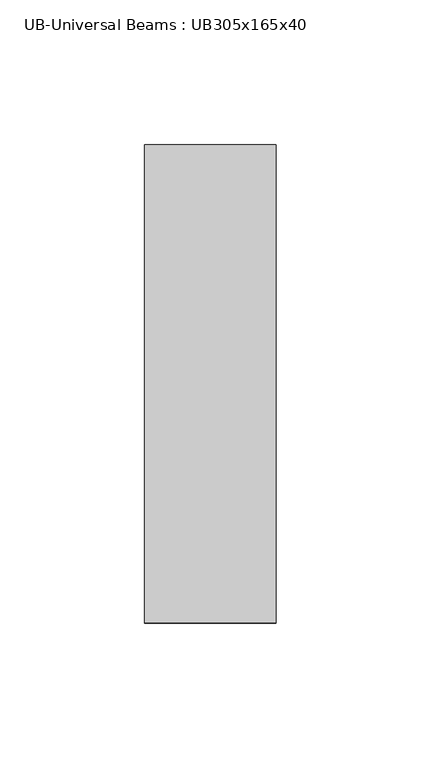
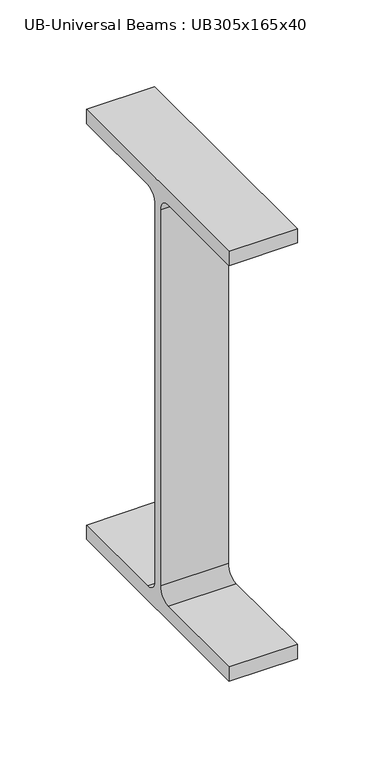
"""IFC4 building model written with IfcOpenShell, lengths in millimetres: beam geometry, UB-Universal Beams : UB305x165x40."""

from ifc_helpers import new_model, si_unit, point, frame, frame_2d, origin, place, context, project, spatial, polyline, circle_curve, trimmed, segment, composite_curve, outline, extrude, source, transform, mapped, element, save


def ub_universal_beams_ub305x165x40_bc9e57b7(model_context):
    return source(origin(), model_context, "Body", "SweptSolid", [
        extrude(outline(composite_curve([segment(polyline([(82.5, -141.5), (82.5, -151.7), (-82.5, -151.7), (-82.5, -141.5), (-11.9, -141.5)]), True, "CONTINUOUS"), segment(trimmed(circle_curve(frame_2d((-11.9, -132.6)), 8.9), [point((-11.9, -141.5))], [point((-3.0, -132.6))], True, "CARTESIAN"), True, "CONTINUOUS"), segment(polyline([(-3.0, -132.6), (-3.0, 132.6)]), True, "CONTINUOUS"), segment(trimmed(circle_curve(frame_2d((-11.9, 132.6)), 8.9), [point((-3.0, 132.6))], [point((-11.9, 141.5))], True, "CARTESIAN"), True, "CONTINUOUS"), segment(polyline([(-11.9, 141.5), (-82.5, 141.5), (-82.5, 151.7), (82.5, 151.7), (82.5, 141.5), (11.9, 141.5)]), True, "CONTINUOUS"), segment(trimmed(circle_curve(frame_2d((11.9, 132.6)), 8.9), [point((11.9, 141.5))], [point((3.0, 132.6))], True, "CARTESIAN"), True, "CONTINUOUS"), segment(polyline([(3.0, 132.6), (3.0, -132.6)]), True, "CONTINUOUS"), segment(trimmed(circle_curve(frame_2d((11.9, -132.6)), 8.9), [point((3.0, -132.6))], [point((11.9, -141.5))], True, "CARTESIAN"), True, "CONTINUOUS"), segment(polyline([(11.9, -141.5), (82.5, -141.5)]), True, "CONTINUOUS")], self_intersect=False)), frame((-35.6, 0.0, 0.0), z_axis=(1.0, 0.0, 0.0), x_axis=(0.0, 1.0, 0.0)), (0.0, 0.0, 1.0), 45.4),
    ])


if __name__ == "__main__":
    model = new_model("IFC4")
    model_context = context("Model", 3, world=origin())
    ifc_project = project(units=[si_unit("LENGTHUNIT", "METRE", prefix="MILLI")], contexts=[model_context])
    site = spatial("IfcSite", under=ifc_project)
    building = spatial("IfcBuilding", under=site)
    placement = place(None, origin())
    ub_universal_beams_ub305x165x40_shape = ub_universal_beams_ub305x165x40_bc9e57b7(model_context)
    element("IfcBeam", 1, ObjectType="UB-Universal Beams : UB305x165x40", at=placement, inside=building, context=model_context, shape_type="MappedRepresentation", body=[
        mapped(ub_universal_beams_ub305x165x40_shape, transform((0.0, 0.0, 0.0), x_axis=(1.0, 0.0, 0.0), y_axis=(0.0, 1.0, 0.0), z_axis=(0.0, 0.0, 1.0))),
    ])
    save(model, "model.ifc")

# Revit data of these elements
# Type "UB-Universal Beams : UB305x165x40"
#   Section Name Key = "UB305X165X40"
#   Width = 16.5 cm
#   Web Thickness = 0.6 cm
#   Web Fillet = 0.89 cm
#   Warping Constant = 164000.0 cm⁶
#   Torsional Moment of Inertia = 14.70 cm⁴
#   Section Area = 51.3 cm²
#   Plastic Modulus weak axis = 142.0 cm³
#   Plastic Modulus strong axis = 623.0 cm³
#   Nominal Weight = 40.2999 kgf/m
#   Moment of Inertia weak axis = 764.00 cm⁴
#   Moment of Inertia strong axis = 8503.00 cm⁴
#   Height = 30.34 cm
#   Flange Thickness = 1.02 cm
#   Elastic Modulus weak axis = 92.6 cm³
#   Elastic Modulus strong axis = 560.0 cm³
#   Centroid Vertical = 15.17 cm
#   Centroid Horizontal = 8.25 cm
#   Bolt Spacing = 9.0 cm
#   Length [instance default] = 1500 mm
#   Structural Material [instance default] = Metal - Steel 43-275
#   Type Comments = ""
#   Assembly Code = ""
# Element 1 (IfcBeam, "UB-Universal Beams : UB305x165x40")
#   Materials on its faces: "Metal - Steel 43-275"
# Materials
#   "Metal - Steel 43-275": class "Metal", colour RGB 247 247 247, transparency 0, Cost = 0
